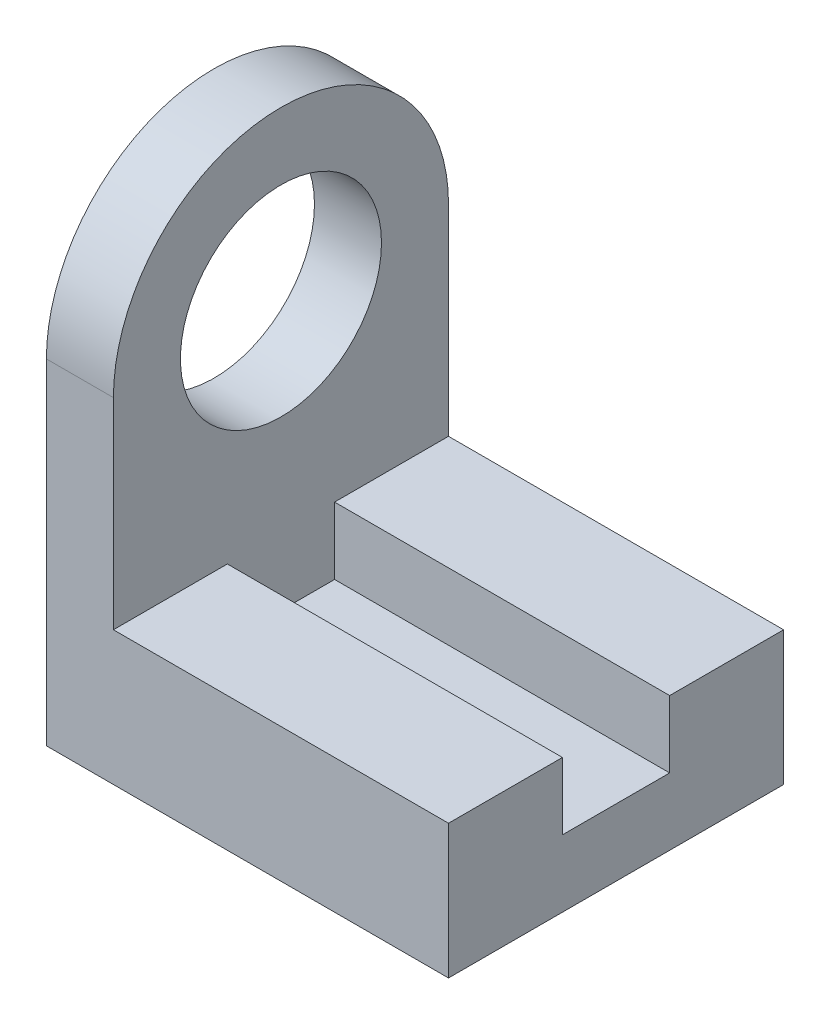
ISO-10303-21;
HEADER;
FILE_DESCRIPTION(('STEP AP214'),'2;1');
FILE_NAME('part.step','',(''),(''),'','','');
FILE_SCHEMA(('AUTOMOTIVE_DESIGN { 1 0 10303 214 1 1 1 1 }'));
ENDSEC;
DATA;
#1=APPLICATION_CONTEXT('core data for automotive mechanical design processes');
#2=APPLICATION_PROTOCOL_DEFINITION('international standard','automotive_design',2000,#1);
#3=PRODUCT_CONTEXT('',#1,'mechanical');
#4=PRODUCT('Part','Part','',(#3));
#5=PRODUCT_RELATED_PRODUCT_CATEGORY('part','',(#4));
#6=PRODUCT_DEFINITION_FORMATION('','',#4);
#7=PRODUCT_DEFINITION_CONTEXT('part definition',#1,'design');
#8=PRODUCT_DEFINITION('design','',#6,#7);
#9=PRODUCT_DEFINITION_SHAPE('','',#8);
#10=(LENGTH_UNIT() NAMED_UNIT(*) SI_UNIT(.MILLI.,.METRE.));
#11=(NAMED_UNIT(*) PLANE_ANGLE_UNIT() SI_UNIT($,.RADIAN.));
#12=(NAMED_UNIT(*) SI_UNIT($,.STERADIAN.) SOLID_ANGLE_UNIT());
#13=UNCERTAINTY_MEASURE_WITH_UNIT(LENGTH_MEASURE(1.E-05),#10,'distance_accuracy_value','');
#14=(GEOMETRIC_REPRESENTATION_CONTEXT(3) GLOBAL_UNCERTAINTY_ASSIGNED_CONTEXT((#13)) GLOBAL_UNIT_ASSIGNED_CONTEXT((#10,
#11,#12)) REPRESENTATION_CONTEXT('',''));
#15=CARTESIAN_POINT('',(0.,0.,0.));
#16=DIRECTION('',(0.,0.,1.));
#17=DIRECTION('',(1.,0.,0.));
#18=AXIS2_PLACEMENT_3D('',#15,#16,#17);
#19=CARTESIAN_POINT('',(0.,20.,0.));
#20=DIRECTION('',(0.,1.,0.));
#21=DIRECTION('',(0.,0.,1.));
#22=AXIS2_PLACEMENT_3D('',#19,#20,#21);
#23=PLANE('',#22);
#24=DIRECTION('',(1.,0.,0.));
#25=VECTOR('',#24,1.);
#26=CARTESIAN_POINT('',(-20.,20.,-8.));
#27=LINE('',#26,#25);
#28=CARTESIAN_POINT('',(-20.,20.,-8.));
#29=VERTEX_POINT('',#28);
#30=CARTESIAN_POINT('',(30.,20.,-8.));
#31=VERTEX_POINT('',#30);
#32=EDGE_CURVE('E207',#29,#31,#27,.T.);
#33=ORIENTED_EDGE('',*,*,#32,.T.);
#34=DIRECTION('',(0.,0.,-1.));
#35=VECTOR('',#34,1.);
#36=CARTESIAN_POINT('',(30.,20.,-25.));
#37=LINE('',#36,#35);
#38=CARTESIAN_POINT('',(30.,20.,-25.));
#39=VERTEX_POINT('',#38);
#40=EDGE_CURVE('E161',#31,#39,#37,.T.);
#41=ORIENTED_EDGE('',*,*,#40,.T.);
#42=DIRECTION('',(-1.,0.,0.));
#43=VECTOR('',#42,1.);
#44=CARTESIAN_POINT('',(-30.,20.,-25.));
#45=LINE('',#44,#43);
#46=CARTESIAN_POINT('',(-20.,20.,-25.));
#47=VERTEX_POINT('',#46);
#48=EDGE_CURVE('E159',#39,#47,#45,.T.);
#49=ORIENTED_EDGE('',*,*,#48,.T.);
#50=DIRECTION('',(0.,0.,-1.));
#51=VECTOR('',#50,1.);
#52=CARTESIAN_POINT('',(-20.,20.,-25.));
#53=LINE('',#52,#51);
#54=EDGE_CURVE('E148',#29,#47,#53,.T.);
#55=ORIENTED_EDGE('',*,*,#54,.F.);
#56=EDGE_LOOP('',(#33,#41,#49,#55));
#57=FACE_BOUND('',#56,.T.);
#58=ADVANCED_FACE('F50',(#57),#23,.T.);
#59=CARTESIAN_POINT('',(30.,20.,-25.));
#60=DIRECTION('',(-1.,0.,0.));
#61=DIRECTION('',(0.,0.,1.));
#62=AXIS2_PLACEMENT_3D('',#59,#60,#61);
#63=PLANE('',#62);
#64=ORIENTED_EDGE('',*,*,#40,.F.);
#65=DIRECTION('',(0.,1.,0.));
#66=VECTOR('',#65,1.);
#67=CARTESIAN_POINT('',(30.,10.,-8.));
#68=LINE('',#67,#66);
#69=CARTESIAN_POINT('',(30.,10.,-8.));
#70=VERTEX_POINT('',#69);
#71=EDGE_CURVE('E132',#70,#31,#68,.T.);
#72=ORIENTED_EDGE('',*,*,#71,.F.);
#73=DIRECTION('',(0.,0.,-1.));
#74=VECTOR('',#73,1.);
#75=CARTESIAN_POINT('',(30.,10.,8.));
#76=LINE('',#75,#74);
#77=CARTESIAN_POINT('',(30.,10.,8.));
#78=VERTEX_POINT('',#77);
#79=EDGE_CURVE('E205',#78,#70,#76,.T.);
#80=ORIENTED_EDGE('',*,*,#79,.F.);
#81=DIRECTION('',(0.,-1.,0.));
#82=VECTOR('',#81,1.);
#83=CARTESIAN_POINT('',(30.,20.,8.));
#84=LINE('',#83,#82);
#85=CARTESIAN_POINT('',(30.,20.,8.));
#86=VERTEX_POINT('',#85);
#87=EDGE_CURVE('E200',#86,#78,#84,.T.);
#88=ORIENTED_EDGE('',*,*,#87,.F.);
#89=CARTESIAN_POINT('',(30.,20.,25.));
#90=VERTEX_POINT('',#89);
#91=EDGE_CURVE('E136',#90,#86,#37,.T.);
#92=ORIENTED_EDGE('',*,*,#91,.F.);
#93=DIRECTION('',(0.,-1.,0.));
#94=VECTOR('',#93,1.);
#95=CARTESIAN_POINT('',(30.,20.,25.));
#96=LINE('',#95,#94);
#97=CARTESIAN_POINT('',(30.,0.,25.));
#98=VERTEX_POINT('',#97);
#99=EDGE_CURVE('E167',#90,#98,#96,.T.);
#100=ORIENTED_EDGE('',*,*,#99,.T.);
#101=DIRECTION('',(0.,0.,-1.));
#102=VECTOR('',#101,1.);
#103=CARTESIAN_POINT('',(30.,0.,-25.));
#104=LINE('',#103,#102);
#105=CARTESIAN_POINT('',(30.,0.,-25.));
#106=VERTEX_POINT('',#105);
#107=EDGE_CURVE('E158',#98,#106,#104,.T.);
#108=ORIENTED_EDGE('',*,*,#107,.T.);
#109=DIRECTION('',(0.,-1.,0.));
#110=VECTOR('',#109,1.);
#111=CARTESIAN_POINT('',(30.,20.,-25.));
#112=LINE('',#111,#110);
#113=EDGE_CURVE('E11',#39,#106,#112,.T.);
#114=ORIENTED_EDGE('',*,*,#113,.F.);
#115=EDGE_LOOP('',(#64,#72,#80,#88,#92,#100,#108,#114));
#116=FACE_BOUND('',#115,.T.);
#117=ADVANCED_FACE('F47',(#116),#63,.F.);
#118=CARTESIAN_POINT('',(-30.,20.,-25.));
#119=DIRECTION('',(0.,0.,1.));
#120=DIRECTION('',(1.,0.,0.));
#121=AXIS2_PLACEMENT_3D('',#118,#119,#120);
#122=PLANE('',#121);
#123=DIRECTION('',(-1.,0.,0.));
#124=VECTOR('',#123,1.);
#125=CARTESIAN_POINT('',(-30.,0.,-25.));
#126=LINE('',#125,#124);
#127=CARTESIAN_POINT('',(-30.,0.,-25.));
#128=VERTEX_POINT('',#127);
#129=EDGE_CURVE('E166',#106,#128,#126,.T.);
#130=ORIENTED_EDGE('',*,*,#129,.T.);
#131=DIRECTION('',(0.,-1.,0.));
#132=VECTOR('',#131,1.);
#133=CARTESIAN_POINT('',(-30.,20.,-25.));
#134=LINE('',#133,#132);
#135=CARTESIAN_POINT('',(-30.,50.,-25.));
#136=VERTEX_POINT('',#135);
#137=EDGE_CURVE('E54',#136,#128,#134,.T.);
#138=ORIENTED_EDGE('',*,*,#137,.F.);
#139=DIRECTION('',(-1.,0.,0.));
#140=VECTOR('',#139,1.);
#141=CARTESIAN_POINT('',(-30.,50.,-25.));
#142=LINE('',#141,#140);
#143=CARTESIAN_POINT('',(-20.,50.,-25.));
#144=VERTEX_POINT('',#143);
#145=EDGE_CURVE('E149',#144,#136,#142,.T.);
#146=ORIENTED_EDGE('',*,*,#145,.F.);
#147=DIRECTION('',(0.,-1.,0.));
#148=VECTOR('',#147,1.);
#149=CARTESIAN_POINT('',(-20.,50.,-25.));
#150=LINE('',#149,#148);
#151=EDGE_CURVE('E152',#144,#47,#150,.T.);
#152=ORIENTED_EDGE('',*,*,#151,.T.);
#153=ORIENTED_EDGE('',*,*,#48,.F.);
#154=ORIENTED_EDGE('',*,*,#113,.T.);
#155=EDGE_LOOP('',(#130,#138,#146,#152,#153,#154));
#156=FACE_BOUND('',#155,.T.);
#157=ADVANCED_FACE('F228',(#156),#122,.F.);
#158=CARTESIAN_POINT('',(-30.,20.,-25.));
#159=DIRECTION('',(1.,0.,0.));
#160=DIRECTION('',(0.,0.,-1.));
#161=AXIS2_PLACEMENT_3D('',#158,#159,#160);
#162=PLANE('',#161);
#163=CARTESIAN_POINT('',(-30.,50.,0.));
#164=DIRECTION('',(1.,0.,0.));
#165=DIRECTION('',(0.,0.,-1.));
#166=AXIS2_PLACEMENT_3D('',#163,#164,#165);
#167=CIRCLE('',#166,15.);
#168=CARTESIAN_POINT('',(-30.,50.,-15.));
#169=VERTEX_POINT('',#168);
#170=EDGE_CURVE('E216',#169,#169,#167,.T.);
#171=ORIENTED_EDGE('',*,*,#170,.T.);
#172=EDGE_LOOP('',(#171));
#173=FACE_BOUND('',#172,.T.);
#174=DIRECTION('',(0.,-1.,0.));
#175=VECTOR('',#174,1.);
#176=CARTESIAN_POINT('',(-30.,20.,25.));
#177=LINE('',#176,#175);
#178=CARTESIAN_POINT('',(-30.,50.,25.));
#179=VERTEX_POINT('',#178);
#180=CARTESIAN_POINT('',(-30.,0.,25.));
#181=VERTEX_POINT('',#180);
#182=EDGE_CURVE('E180',#179,#181,#177,.T.);
#183=ORIENTED_EDGE('',*,*,#182,.F.);
#184=CARTESIAN_POINT('',(-30.,50.,0.));
#185=DIRECTION('',(1.,0.,0.));
#186=DIRECTION('',(0.,0.,-1.));
#187=AXIS2_PLACEMENT_3D('',#184,#185,#186);
#188=CIRCLE('',#187,25.);
#189=EDGE_CURVE('E151',#136,#179,#188,.T.);
#190=ORIENTED_EDGE('',*,*,#189,.F.);
#191=ORIENTED_EDGE('',*,*,#137,.T.);
#192=DIRECTION('',(0.,0.,1.));
#193=VECTOR('',#192,1.);
#194=CARTESIAN_POINT('',(-30.,0.,-25.));
#195=LINE('',#194,#193);
#196=EDGE_CURVE('E173',#128,#181,#195,.T.);
#197=ORIENTED_EDGE('',*,*,#196,.T.);
#198=EDGE_LOOP('',(#183,#190,#191,#197));
#199=FACE_BOUND('',#198,.T.);
#200=ADVANCED_FACE('F181',(#173,#199),#162,.F.);
#201=CARTESIAN_POINT('',(-30.,20.,25.));
#202=DIRECTION('',(0.,0.,-1.));
#203=DIRECTION('',(-1.,0.,0.));
#204=AXIS2_PLACEMENT_3D('',#201,#202,#203);
#205=PLANE('',#204);
#206=DIRECTION('',(1.,0.,0.));
#207=VECTOR('',#206,1.);
#208=CARTESIAN_POINT('',(-30.,0.,25.));
#209=LINE('',#208,#207);
#210=EDGE_CURVE('E172',#181,#98,#209,.T.);
#211=ORIENTED_EDGE('',*,*,#210,.T.);
#212=ORIENTED_EDGE('',*,*,#99,.F.);
#213=DIRECTION('',(1.,0.,0.));
#214=VECTOR('',#213,1.);
#215=CARTESIAN_POINT('',(-30.,20.,25.));
#216=LINE('',#215,#214);
#217=CARTESIAN_POINT('',(-20.,20.,25.));
#218=VERTEX_POINT('',#217);
#219=EDGE_CURVE('E163',#218,#90,#216,.T.);
#220=ORIENTED_EDGE('',*,*,#219,.F.);
#221=DIRECTION('',(0.,-1.,0.));
#222=VECTOR('',#221,1.);
#223=CARTESIAN_POINT('',(-20.,50.,25.));
#224=LINE('',#223,#222);
#225=CARTESIAN_POINT('',(-20.,50.,25.));
#226=VERTEX_POINT('',#225);
#227=EDGE_CURVE('E145',#226,#218,#224,.T.);
#228=ORIENTED_EDGE('',*,*,#227,.F.);
#229=DIRECTION('',(1.,0.,0.));
#230=VECTOR('',#229,1.);
#231=CARTESIAN_POINT('',(-20.,50.,25.));
#232=LINE('',#231,#230);
#233=EDGE_CURVE('E144',#179,#226,#232,.T.);
#234=ORIENTED_EDGE('',*,*,#233,.F.);
#235=ORIENTED_EDGE('',*,*,#182,.T.);
#236=EDGE_LOOP('',(#211,#212,#220,#228,#234,#235));
#237=FACE_BOUND('',#236,.T.);
#238=ADVANCED_FACE('F191',(#237),#205,.F.);
#239=DIRECTION('',(1.,0.,0.));
#240=VECTOR('',#239,1.);
#241=CARTESIAN_POINT('',(-20.,20.,8.));
#242=LINE('',#241,#240);
#243=CARTESIAN_POINT('',(-20.,20.,8.));
#244=VERTEX_POINT('',#243);
#245=EDGE_CURVE('E126',#244,#86,#242,.T.);
#246=ORIENTED_EDGE('',*,*,#245,.F.);
#247=EDGE_CURVE('E67',#218,#244,#53,.T.);
#248=ORIENTED_EDGE('',*,*,#247,.F.);
#249=ORIENTED_EDGE('',*,*,#219,.T.);
#250=ORIENTED_EDGE('',*,*,#91,.T.);
#251=EDGE_LOOP('',(#246,#248,#249,#250));
#252=FACE_BOUND('',#251,.T.);
#253=ADVANCED_FACE('F138',(#252),#23,.T.);
#254=CARTESIAN_POINT('',(0.,0.,0.));
#255=DIRECTION('',(0.,1.,0.));
#256=DIRECTION('',(0.,0.,1.));
#257=AXIS2_PLACEMENT_3D('',#254,#255,#256);
#258=PLANE('',#257);
#259=ORIENTED_EDGE('',*,*,#107,.F.);
#260=ORIENTED_EDGE('',*,*,#210,.F.);
#261=ORIENTED_EDGE('',*,*,#196,.F.);
#262=ORIENTED_EDGE('',*,*,#129,.F.);
#263=EDGE_LOOP('',(#259,#260,#261,#262));
#264=FACE_BOUND('',#263,.T.);
#265=ADVANCED_FACE('F186',(#264),#258,.F.);
#266=CARTESIAN_POINT('',(-20.,50.,-25.));
#267=DIRECTION('',(-1.,0.,0.));
#268=DIRECTION('',(0.,0.,1.));
#269=AXIS2_PLACEMENT_3D('',#266,#267,#268);
#270=PLANE('',#269);
#271=CARTESIAN_POINT('',(-20.,50.,0.));
#272=DIRECTION('',(1.,0.,0.));
#273=DIRECTION('',(0.,0.,-1.));
#274=AXIS2_PLACEMENT_3D('',#271,#272,#273);
#275=CIRCLE('',#274,15.);
#276=CARTESIAN_POINT('',(-20.,50.,-15.));
#277=VERTEX_POINT('',#276);
#278=EDGE_CURVE('E215',#277,#277,#275,.T.);
#279=ORIENTED_EDGE('',*,*,#278,.F.);
#280=EDGE_LOOP('',(#279));
#281=FACE_BOUND('',#280,.T.);
#282=ORIENTED_EDGE('',*,*,#151,.F.);
#283=CARTESIAN_POINT('',(-20.,50.,0.));
#284=DIRECTION('',(1.,0.,0.));
#285=DIRECTION('',(0.,0.,-1.));
#286=AXIS2_PLACEMENT_3D('',#283,#284,#285);
#287=CIRCLE('',#286,25.);
#288=EDGE_CURVE('E218',#144,#226,#287,.T.);
#289=ORIENTED_EDGE('',*,*,#288,.T.);
#290=ORIENTED_EDGE('',*,*,#227,.T.);
#291=ORIENTED_EDGE('',*,*,#247,.T.);
#292=DIRECTION('',(0.,-1.,0.));
#293=VECTOR('',#292,1.);
#294=CARTESIAN_POINT('',(-20.,20.,8.));
#295=LINE('',#294,#293);
#296=CARTESIAN_POINT('',(-20.,10.,8.));
#297=VERTEX_POINT('',#296);
#298=EDGE_CURVE('E122',#244,#297,#295,.T.);
#299=ORIENTED_EDGE('',*,*,#298,.T.);
#300=DIRECTION('',(0.,0.,-1.));
#301=VECTOR('',#300,1.);
#302=CARTESIAN_POINT('',(-20.,10.,8.));
#303=LINE('',#302,#301);
#304=CARTESIAN_POINT('',(-20.,10.,-8.));
#305=VERTEX_POINT('',#304);
#306=EDGE_CURVE('E134',#297,#305,#303,.T.);
#307=ORIENTED_EDGE('',*,*,#306,.T.);
#308=DIRECTION('',(0.,1.,0.));
#309=VECTOR('',#308,1.);
#310=CARTESIAN_POINT('',(-20.,10.,-8.));
#311=LINE('',#310,#309);
#312=EDGE_CURVE('E64',#305,#29,#311,.T.);
#313=ORIENTED_EDGE('',*,*,#312,.T.);
#314=ORIENTED_EDGE('',*,*,#54,.T.);
#315=EDGE_LOOP('',(#282,#289,#290,#291,#299,#307,#313,#314));
#316=FACE_BOUND('',#315,.T.);
#317=ADVANCED_FACE('F142',(#281,#316),#270,.F.);
#318=CARTESIAN_POINT('',(-30.,50.,0.));
#319=DIRECTION('',(1.,0.,0.));
#320=DIRECTION('',(0.,0.,-1.));
#321=AXIS2_PLACEMENT_3D('',#318,#319,#320);
#322=CYLINDRICAL_SURFACE('',#321,25.);
#323=ORIENTED_EDGE('',*,*,#145,.T.);
#324=ORIENTED_EDGE('',*,*,#189,.T.);
#325=ORIENTED_EDGE('',*,*,#233,.T.);
#326=ORIENTED_EDGE('',*,*,#288,.F.);
#327=EDGE_LOOP('',(#323,#324,#325,#326));
#328=FACE_BOUND('',#327,.T.);
#329=ADVANCED_FACE('F223',(#328),#322,.T.);
#330=CARTESIAN_POINT('',(-30.,50.,0.));
#331=DIRECTION('',(1.,0.,0.));
#332=DIRECTION('',(0.,0.,-1.));
#333=AXIS2_PLACEMENT_3D('',#330,#331,#332);
#334=CYLINDRICAL_SURFACE('',#333,15.);
#335=ORIENTED_EDGE('',*,*,#170,.F.);
#336=EDGE_LOOP('',(#335));
#337=FACE_BOUND('',#336,.T.);
#338=ORIENTED_EDGE('',*,*,#278,.T.);
#339=EDGE_LOOP('',(#338));
#340=FACE_BOUND('',#339,.T.);
#341=ADVANCED_FACE('F243',(#337,#340),#334,.F.);
#342=CARTESIAN_POINT('',(-20.,10.,-8.));
#343=DIRECTION('',(0.,0.,-1.));
#344=DIRECTION('',(-1.,0.,0.));
#345=AXIS2_PLACEMENT_3D('',#342,#343,#344);
#346=PLANE('',#345);
#347=ORIENTED_EDGE('',*,*,#71,.T.);
#348=ORIENTED_EDGE('',*,*,#32,.F.);
#349=ORIENTED_EDGE('',*,*,#312,.F.);
#350=DIRECTION('',(1.,0.,0.));
#351=VECTOR('',#350,1.);
#352=CARTESIAN_POINT('',(-20.,10.,-8.));
#353=LINE('',#352,#351);
#354=EDGE_CURVE('E213',#305,#70,#353,.T.);
#355=ORIENTED_EDGE('',*,*,#354,.T.);
#356=EDGE_LOOP('',(#347,#348,#349,#355));
#357=FACE_BOUND('',#356,.T.);
#358=ADVANCED_FACE('F233',(#357),#346,.F.);
#359=CARTESIAN_POINT('',(-20.,10.,8.));
#360=DIRECTION('',(0.,-1.,0.));
#361=DIRECTION('',(0.,0.,-1.));
#362=AXIS2_PLACEMENT_3D('',#359,#360,#361);
#363=PLANE('',#362);
#364=ORIENTED_EDGE('',*,*,#79,.T.);
#365=ORIENTED_EDGE('',*,*,#354,.F.);
#366=ORIENTED_EDGE('',*,*,#306,.F.);
#367=DIRECTION('',(1.,0.,0.));
#368=VECTOR('',#367,1.);
#369=CARTESIAN_POINT('',(-20.,10.,8.));
#370=LINE('',#369,#368);
#371=EDGE_CURVE('E128',#297,#78,#370,.T.);
#372=ORIENTED_EDGE('',*,*,#371,.T.);
#373=EDGE_LOOP('',(#364,#365,#366,#372));
#374=FACE_BOUND('',#373,.T.);
#375=ADVANCED_FACE('F231',(#374),#363,.F.);
#376=CARTESIAN_POINT('',(-20.,20.,8.));
#377=DIRECTION('',(0.,0.,1.));
#378=DIRECTION('',(0.,-1.,0.));
#379=AXIS2_PLACEMENT_3D('',#376,#377,#378);
#380=PLANE('',#379);
#381=ORIENTED_EDGE('',*,*,#87,.T.);
#382=ORIENTED_EDGE('',*,*,#371,.F.);
#383=ORIENTED_EDGE('',*,*,#298,.F.);
#384=ORIENTED_EDGE('',*,*,#245,.T.);
#385=EDGE_LOOP('',(#381,#382,#383,#384));
#386=FACE_BOUND('',#385,.T.);
#387=ADVANCED_FACE('F130',(#386),#380,.F.);
#388=CLOSED_SHELL('',(#58,#117,#157,#200,#238,#253,#265,#317,#329,#341,#358,#375,#387));
#389=MANIFOLD_SOLID_BREP('B2',#388);
#390=ADVANCED_BREP_SHAPE_REPRESENTATION('',(#18,#389),#14);
#391=SHAPE_DEFINITION_REPRESENTATION(#9,#390);
ENDSEC;
END-ISO-10303-21;
